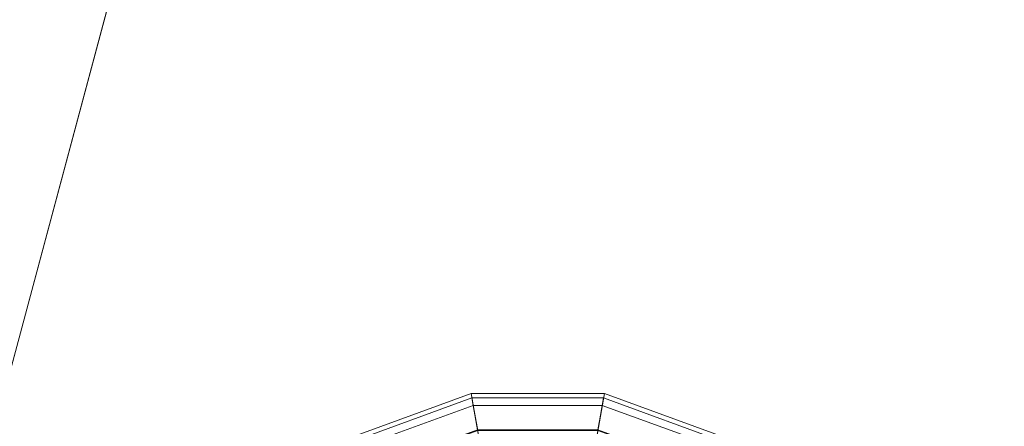
# Model space of a CAD drawing. Units: inches. Extents: x 375 to 1122, y 27 to 1069.
# Tile 101 of 155: x 717.434 to 720.91, y 866.486 to 867.921. Entities that reach past the tile are written whole.
import ezdxf

# ---------------------------------------------------------------- set-up
doc = ezdxf.new("R2010")
doc.units = ezdxf.units.IN
doc.layers.add('A-ANNO-DIMS', color=2, linetype='Continuous', lineweight=18)
doc.layers.add('Furniture', color=30, linetype='Continuous', lineweight=18)
doc.styles.get("Standard").update_dxf_attribs({"font": 'arial.ttf'})
doc.dimstyles.new('ISO-25', dxfattribs={"dimtxt": 12, "dimasz": 2.5, "dimexe": 1.5, "dimexo": 1.5, "dimtad": 1, "dimdec": 1, "dimlunit": 3, "dimtxsty": 'Standard', "dimblk": 'ARCHTICK', "dimcen": 2.5, "dimadec": 0, "dimazin": 0, "dimtfac": 1, "dimtdec": 1, "dimtmove": 0, "dimatfit": 3, "dimfxl": 1.5, "dimfxlon": 1, "dimarcsym": 0})

# ---------------------------------------------------------------- blocks, each defined once
blk = doc.blocks.new('A$C403C54AD')
for points in [[(1.800062, 0.873182, -0.028594), (1.797233, 0.874815, -0.031825), (1.793211, 0.863764, -0.031825), (1.796427, 0.863197, -0.028594)], [(1.797233, 0.874815, -0.031825), (1.826559, 0.857884, -0.028747), (1.826559, 0.857884, -0.028747), (1.793211, 0.863764, -0.031825)], [(1.800097, 0.873162, 0.131159), (1.797579, 0.874616, 0.117935), (1.793604, 0.863695, 0.117935), (1.796467, 0.86319, 0.131159)], [(1.797579, 0.874616, 0.117935), (1.798163, 0.874278, 0.089693), (1.794269, 0.863578, 0.089693), (1.793604, 0.863695, 0.117935)], [(1.798163, 0.874278, 0.089693), (1.802809, 0.871596, 0.071684), (1.799552, 0.862646, 0.071684), (1.794269, 0.863578, 0.089693)], [(1.796427, 0.863197, -0.028594), (1.793211, 0.863764, -0.031825), (1.793211, 0.852004, -0.031825), (1.796427, 0.852571, -0.028594)], [(1.793211, 0.863764, -0.031825), (1.826559, 0.857884, -0.028747), (1.826559, 0.857884, -0.028747), (1.793211, 0.852004, -0.031825)], [(1.796467, 0.86319, 0.131159), (1.793604, 0.863695, 0.117935), (1.793604, 0.852073, 0.117935), (1.796467, 0.852578, 0.131159)], [(1.793604, 0.863695, 0.117935), (1.794269, 0.863578, 0.089693), (1.794269, 0.85219, 0.089693), (1.793604, 0.852073, 0.117935)], [(1.794269, 0.863578, 0.089693), (1.799552, 0.862646, 0.071684), (1.799552, 0.853122, 0.071684), (1.794269, 0.85219, 0.089693)], [(1.793211, 0.852004, -0.031825), (1.826559, 0.857884, -0.028747), (1.826559, 0.857884, -0.028747), (1.797233, 0.840953, -0.031825)], [(1.794269, 0.85219, 0.089693), (1.799552, 0.853122, 0.071684), (1.802809, 0.844172, 0.071684), (1.798163, 0.84149, 0.089693)], [(1.796427, 0.852571, -0.028594), (1.793211, 0.852004, -0.031825), (1.797233, 0.840953, -0.031825), (1.800062, 0.842586, -0.028594)], [(1.796467, 0.852578, 0.131159), (1.793604, 0.852073, 0.117935), (1.797579, 0.841152, 0.117935), (1.800097, 0.842606, 0.131159)], [(1.793604, 0.852073, 0.117935), (1.794269, 0.85219, 0.089693), (1.798163, 0.84149, 0.089693), (1.797579, 0.841152, 0.117935)]]:
    blk.add_3dface(points)
at = {"linetype": 'ByBlock', "invisible_edges": 5}
for points in [[(1.795775, 0.81008, -0.008737), (1.78654, 0.794084, -0.008737), (1.726512, 0.810169, -0.008737), (1.726512, 0.828639, -0.008737)], [(1.778844, 0.780755, -0.02259), (1.795775, 0.81008, -0.013355), (1.726512, 0.828639, -0.013355), (1.726512, 0.794777, -0.02259)]]:
    blk.add_3dface(points, dxfattribs=at)
at = {"linetype": 'ByBlock'}
blk.add_3dface([(1.795775, 0.81008, -0.013355), (1.795775, 0.81008, -0.008737), (1.726512, 0.828639, -0.008737), (1.726512, 0.828639, -0.013355)], dxfattribs=at)
blk = doc.blocks.new('_ArchTick')
at = {"color": 0, "linetype": 'ByBlock', "const_width": 0.15}
blk.add_lwpolyline([(-0.5, -0.5), (0.5, 0.5)], dxfattribs=at)
blk = doc.blocks.new('*D85')
at = {"layer": 'A-ANNO-DIMS', "color": 0, "lineweight": -2, "transparency": 16777216}
for p, q in [((401.5073, 868.5277), (398.5073, 868.5277)), ((400.0073, 814.5277), (400.0073, 868.5277)), ((401.5073, 814.5277), (398.5073, 814.5277))]:
    blk.add_line(p, q, dxfattribs=at)
at = {"layer": 'Defpoints', "color": 0, "transparency": 16777216}
for p in [(400.0073, 868.5277), (845.0073, 868.5277), (845.0073, 814.5277)]:
    blk.add_point(p, dxfattribs=at)
at = {"layer": 'A-ANNO-DIMS', "color": 0, "lineweight": -2, "transparency": 16777216, "xscale": 2.5, "yscale": 2.5, "zscale": 2.5}
for p, rotation in [((400.0073, 868.5277), 90), ((400.0073, 814.5277), 270)]:
    blk.add_blockref('_ArchTick', p, dxfattribs=dict(at, rotation=rotation))
at = {"layer": 'A-ANNO-DIMS', "color": 0, "transparency": 16777216, "insert": (393.2555, 841.5277), "char_height": 12, "attachment_point": 5, "rotation": 90}
blk.add_mtext('4\'-6"', dxfattribs=at)

msp = doc.modelspace()

# ---------------------------------------------------------------- block references
at = {"layer": 'Furniture', "xscale": 39.9918517141215, "yscale": 39.9918517141215, "zscale": 39.9918517141215, "rotation": 270}
msp.add_blockref('A$C403C54AD', (684.9549, 938.3156, 0.024), dxfattribs=at)

# ---------------------------------------------------------------- dimensions: what is measured, and where the dimension line sits
at = {"layer": 'A-ANNO-DIMS'}
dim = msp.add_linear_dim(base=(400.0073, 868.5277), p1=(845.0073, 814.5277), p2=(845.0073, 868.5277), angle=90, dimstyle='ISO-25', override={"dimdec": 1, "dimlfac": 1, "dimrnd": 0, "dimzin": 1, "dimdsep": 46, "dimlunit": 4, "dimfrac": 2}, dxfattribs=at)
dim.commit()
dim.dimension.update_dxf_attribs({"geometry": '*D85', "text_midpoint": (393.2555, 841.5277)})

doc.saveas('drawing.dxf')
